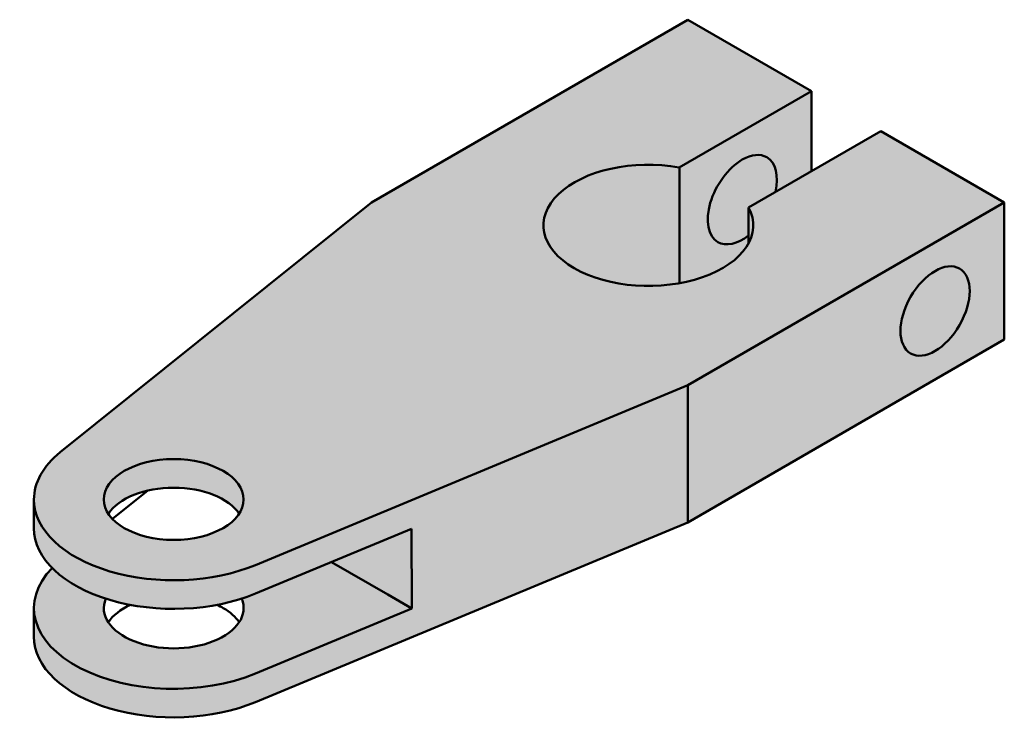
# Model space of a CAD drawing. Units: millimetres. Extents: x 53.2 to 139.4, y -0.6 to 60.9.
import ezdxf

# ---------------------------------------------------------------- set-up
doc = ezdxf.new("R2010")
doc.units = ezdxf.units.MM
doc.header["$MEASUREMENT"] = 0
doc.layers.add('M-HATC', color=18, linetype='Continuous', lineweight=18)
doc.layers.add('M-OUTL', color=18, linetype='Continuous', lineweight=50)

msp = doc.modelspace()

# ---------------------------------------------------------------- hatches: boundary and pattern name
at = {"layer": 'M-HATC'}
h = msp.add_hatch(color=256, dxfattribs=at)
h.dxf.hatch_style = 1
h.set_gradient(color1=(41, 49, 137), color2=(206, 204, 230), tint=1)
edge = h.paths.add_edge_path()
edge.add_line((139.4098702946091, 44.88844877763933), (128.5845527473036, 51.13844877763934))
edge.add_line((128.5845527473036, 51.13844877763934), (117.0086073181529, 44.45507356799473))
edge.add_ellipse((108.2329557583693, 42.88844877763934), major_axis=(-9.185586535436917, 0), ratio=0.577350269189626, start_angle=241.82834790261938, end_angle=550.1217874100114, ccw=False)
edge.add_line((110.9464294916618, 47.95507356799474), (122.5223749208125, 54.63844877763934))
edge.add_line((122.5223749208125, 54.63844877763934), (111.6970573735071, 60.88844877763933))
edge.add_line((111.6970573735071, 60.88844877763933), (83.98424445240506, 44.88844877763933))
edge.add_line((83.98424445240506, 44.88844877763933), (111.6970573735071, 28.88844877763934))
edge.add_line((111.6970573735071, 28.88844877763934), (139.4098702946091, 44.88844877763933))
edge = h.paths.add_edge_path(flags=17)
edge.add_ellipse((108.2329557583693, 42.88844877763934), major_axis=(-9.185586535436917, 0), ratio=0.577350269189626, start_angle=241.8283479026194, end_angle=190.1217874100114)
edge.add_line((117.0086073181529, 44.45507356799473), (122.5223749208125, 47.63844877763934))
edge.add_line((122.5223749208125, 47.63844877763934), (122.5223749208125, 54.63844877763934))
edge.add_line((122.5223749208125, 54.63844877763934), (110.9464294916618, 47.95507356799474))
edge = h.paths.add_edge_path()
edge.add_line((111.6970573735071, 28.88844877763934), (83.98424445240506, 44.88844877763933))
edge.add_line((83.98424445240506, 44.88844877763933), (56.72304746406734, 23.01893316981172))
edge.add_ellipse((66.66373637671627, 18.88844877763934), major_axis=(-12.24744871391589, 0), ratio=0.577350269189626, start_angle=141.2626679741719, end_angle=337.4364855105821, ccw=False)
edge.add_line((73.81794520382898, 13.14918935799111), (111.6970573735071, 28.88844877763934))
edge = h.paths.add_edge_path(flags=17)
edge.add_ellipse((66.66373637671627, 18.88844877763934), major_axis=(-12.24744871391589, 0), ratio=0.577350269189626, start_angle=141.2626679741719, end_angle=337.4364855105821)
edge.add_ellipse((66.66373637671627, 18.88844877763934), major_axis=(-12.24744871391589, 0), ratio=0.577350269189626, start_angle=337.4364855105821, end_angle=360)
edge.add_ellipse((66.66373637671627, 18.88844877763934), major_axis=(-12.24744871391589, 0), ratio=0.577350269189626, start_angle=0, end_angle=141.2626679741719)
edge = h.paths.add_edge_path(flags=17)
edge.add_ellipse((66.66373637671627, 18.88844877763934), major_axis=(-6.123724356957945, 0), ratio=0.577350269189626, start_angle=167.6900113356715, end_angle=372.30998866432856, ccw=False)
edge.add_ellipse((66.66373637671627, 18.88844877763934), major_axis=(-6.123724356957945, 0), ratio=0.577350269189626, start_angle=12.309988664328614, end_angle=167.6900113356715, ccw=False)
edge = h.paths.add_edge_path(flags=16)
edge.add_ellipse((66.66373637671627, 18.88844877763934), major_axis=(-6.123724356957945, 0), ratio=0.577350269189626, start_angle=167.6900113356714, end_angle=372.3099886643285)
edge.add_ellipse((66.66373637671627, 16.38844877763934), major_axis=(-6.123724356957945, 0), ratio=0.577350269189626, start_angle=192.3099886643286, end_angle=347.69001133567144, ccw=False)
edge = h.paths.add_edge_path()
edge.add_line((111.6970573735071, 16.88844877763934), (111.6970573735071, 28.88844877763934))
edge.add_line((111.6970573735071, 28.88844877763934), (73.81794520382905, 13.14918935799114))
edge.add_ellipse((66.66373637671627, 18.88844877763934), major_axis=(-12.24744871391589, 0), ratio=0.577350269189626, start_angle=0, end_angle=141.2626679741719, ccw=False)
edge.add_line((54.41628766280039, 18.88844877763927), (54.41628766280038, 16.38844877763936))
edge.add_ellipse((66.66373637671627, 16.38844877763934), major_axis=(-12.24744871391589, 0), ratio=0.577350269189626, start_angle=360, end_angle=378.2054506641616)
edge.add_ellipse((66.66373637671627, 16.38844877763934), major_axis=(-12.24744871391589, 0), ratio=0.577350269189626, start_angle=378.2054506641616, end_angle=406.050059065898)
edge.add_ellipse((66.66373637671627, 16.38844877763934), major_axis=(-12.24744871391589, 0), ratio=0.577350269189626, start_angle=406.050059065898, end_angle=493.9499409340927)
edge.add_ellipse((66.66373637671627, 16.38844877763934), major_axis=(-12.24744871391589, 0), ratio=0.577350269189626, start_angle=493.9499409340927, end_angle=501.2626679741718)
edge.add_line((73.81794520382928, 10.64918935799121), (87.49435830124096, 16.3319153074856))
edge.add_line((87.49435830124096, 16.3319153074856), (87.52454201218212, 9.344457028490641))
edge.add_line((87.52454201218212, 9.344457028490641), (73.81794520382905, 3.649189357991133))
edge.add_ellipse((66.66373637671627, 9.388448777639342), major_axis=(-12.24744871391589, 0), ratio=0.577350269189626, start_angle=360.0000000000001, end_angle=501.2626679741719, ccw=False)
edge.add_line((54.41628766280037, 9.388448777639486), (54.41628766280038, 6.888448777639279))
edge.add_ellipse((66.66373637671624, 6.888448777639336), major_axis=(-12.24744871391589, 0), ratio=0.577350269189626, start_angle=360, end_angle=501.2626679741718)
edge.add_line((73.81794520382921, 1.149189357991197), (111.6970573735071, 16.88844877763934))
h.paths.add_polyline_path([(87.49435830124096, 16.3319153074856), (80.47422503179573, 13.41495943498892), (85.42162037359753, 10.55857940261214), (87.52454201218212, 9.344457028490657)], flags=17)
h.paths.add_polyline_path([(139.4098702946091, 32.88844877763934), (139.4098702946091, 44.88844877763933), (111.6970573735071, 28.88844877763935), (111.6970573735071, 16.88844877763934)])
edge = h.paths.add_edge_path(flags=17)
edge.add_line((85.42162037359753, 10.55857940261214), (80.47422503179571, 13.41495943498892))
edge.add_line((80.47422503179571, 13.41495943498892), (73.81794520383022, 10.64918935799158))
edge.add_ellipse((66.66373637671627, 16.38844877763934), major_axis=(-12.24744871391589, 0), ratio=0.577350269189626, start_angle=493.9499409340927, end_angle=501.2626679741719, ccw=False)
edge.add_ellipse((66.66373637671627, 9.388448777639342), major_axis=(-6.123724356957945, 0), ratio=0.577350269189626, start_angle=352.1477236987654, end_angle=547.8522763012346, ccw=False)
edge.add_ellipse((66.66373637671627, 16.38844877763934), major_axis=(-12.24744871391589, 0), ratio=0.577350269189626, start_angle=378.2054506641616, end_angle=406.05005906589804, ccw=False)
edge.add_ellipse((66.66373637671627, 9.388448777639342), major_axis=(-12.24744871391589, 0), ratio=0.577350269189626, start_angle=341.7945493358378, end_angle=360)
edge.add_ellipse((66.66373637671627, 9.388448777639342), major_axis=(-12.24744871391589, 0), ratio=0.577350269189626, start_angle=360, end_angle=501.2626679741718)
edge.add_line((73.81794520382928, 3.649189357991232), (87.52454201218215, 9.344457028490648))
edge.add_line((87.52454201218215, 9.344457028490648), (85.42162037359753, 10.55857940261214))

# ---------------------------------------------------------------- linework, layer by layer
at = {"layer": 'M-OUTL'}
for p, q in [((111.6970573735071, 60.88844877763933), (83.98424445240506, 44.88844877763933)), ((111.6970573735071, 60.88844877763933), (122.5223749208125, 54.63844877763935)), ((122.5223749208125, 54.63844877763934), (110.9464294916618, 47.95507356799474)), ((122.5223749208125, 54.63844877763934), (122.5223749208125, 47.63844877763932)), ((128.5845527473036, 51.13844877763934), (117.0086073181529, 44.45507356799473)), ((128.5845527473036, 51.13844877763934), (139.4098702946091, 44.88844877763933)), ((110.9467306220602, 37.82137520964461), (110.9467306220602, 47.9546247903554)), ((83.98424445240506, 44.88844877763933), (56.72304746406735, 23.01893316981172)), ((139.4098702946091, 44.88844877763933), (111.6970573735071, 28.88844877763934)), ((139.4098702946091, 44.88844877763933), (139.4098702946091, 32.88844877763934)), ((117.0089084485513, 41.32137520964461), (117.0089084485513, 44.45462479035539)), ((111.6970573735071, 16.88844877763934), (139.4098702946091, 32.88844877763934)), ((111.6970573735071, 28.88844877763934), (73.81794520382908, 13.14918935799115)), ((111.6970573735071, 16.88844877763934), (111.6970573735071, 28.88844877763934)), ((111.6970573735071, 22.88844877763934), (111.6970573735071, 26.38844877763934)), ((111.6970573735071, 22.88844877763934), (111.6970573735071, 19.38844877763934)), ((61.29591728248195, 17.18669802270061), (64.39329454675568, 19.67148018663023)), ((54.41628766280039, 16.38844877763934), (54.41628766280039, 18.88844877763934)), ((111.697057373507, 16.88844877763933), (73.81794520382907, 1.149189357991151)), ((87.49435830124095, 16.33191530748559), (73.81794520382908, 10.64918935799115)), ((87.52454201218212, 9.344457028490636), (87.49435830124096, 16.33191530748559)), ((80.4742250317957, 13.41495943498894), (85.42162037359753, 10.55857940261214)), ((85.42162037359753, 10.55857940261214), (87.52454201218215, 9.344457028490641)), ((54.41628766280037, 6.888448777639336), (54.41628766280036, 9.38844877763933)), ((87.52454201218212, 9.344457028490645), (73.81794520382905, 3.649189357991143)), ((87.52454201218215, 9.344457028490645), (73.81794520382908, 3.649189357991157))]:
    msp.add_line(p, q, dxfattribs=at)
for centre, major_axis, ratio, start_param, end_param in [((116.4604982247199, 45.13800000000001), (2.14330352493528, 3.712310601229374), 0.5773502691896257, 2e-16, 0.7853981633974485), ((108.2329557583693, 42.88844877763934), (-9.185586535436917, 0), 0.577350269189626, 4.412508939282832, 9.724658001871235), ((116.4604982247199, 45.13800000000001), (2.14330352493528, 3.712310601229374), 0.5773502691896257, 0.7853981633974485, 3.141592653589793), ((116.4604982247199, 45.13800000000001), (2.14330352493528, 3.712310601229374), 0.5773502691896257, 5.208035442346089, 6.283185307179586), ((116.4604982247199, 45.13800000000001), (2.14330352493528, 3.712310601229374), 0.5773502691896257, 3.141592653589793, 4.108921218098146), ((66.66403871285326, 18.88800069613347), (-12.24745041908766, -5e-16), 0.577350269189626, 5.659366931634969, 6.283185307179586), ((66.66373637671627, 16.38844877763934), (-6.123724356957945, 0), 0.577350269189626, 3.502959777496501, 5.921818183272878), ((66.66403871285326, 18.88800069613347), (-12.24745041908766, -5e-16), 0.577350269189626, 2e-16, 2.194614702339513), ((66.66373637671627, 16.38844877763934), (-12.24744871391589, 0), 0.577350269189626, 6.283185307179586, 8.477800125105336), ((66.66373637671624, 9.38844877763933), (-12.24744871391589, 0), 0.577350269189626, 5.765379538919934, 8.477800125105336), ((66.66373637671627, 9.388448777639342), (-12.24744871391589, 0), 0.577350269189626, 5.765379538919937, 8.477800125105336), ((66.66373637671624, 9.38844877763933), (-6.123724356957945, 0), 0.577350269189626, 6.048707529338069, 9.659255738610891), ((66.66373637671627, 9.388448777639342), (-6.123724356957945, 0), 0.577350269189626, 6.048707529338074, 9.659255738610891), ((66.66403750711474, 6.888000000000002), (6.123724356957945, -3e-16), 0.577350269189626, 2.23847564299005, 2.780225529683085), ((66.66403750711474, 6.888000000000002), (6.123724356957945, -3e-16), 0.577350269189626, 0.7853981633974482, 0.9031168640453396), ((66.66403750711474, 6.888000000000002), (6.123724356957945, -3e-16), 0.577350269189626, 0.3613671239067075, 0.7853981633974482), ((66.66373637671624, 6.888448777639336), (-12.24744871391589, 0), 0.577350269189626, 6.283185307179586, 8.477800125105336)]:
    msp.add_ellipse(centre, major_axis=major_axis, ratio=ratio, start_param=start_param, end_param=end_param, dxfattribs=at)
for centre, major_axis, ratio in [((133.347692468118, 35.38844877763934), (-2.143303524935287, -3.712310601229369), 0.5773502691896254), ((66.66373637671627, 18.88844877763934), (-6.123724356957945, 0), 0.577350269189626)]:
    msp.add_ellipse(centre, major_axis=major_axis, ratio=ratio, dxfattribs=at)

doc.saveas('drawing.dxf')
